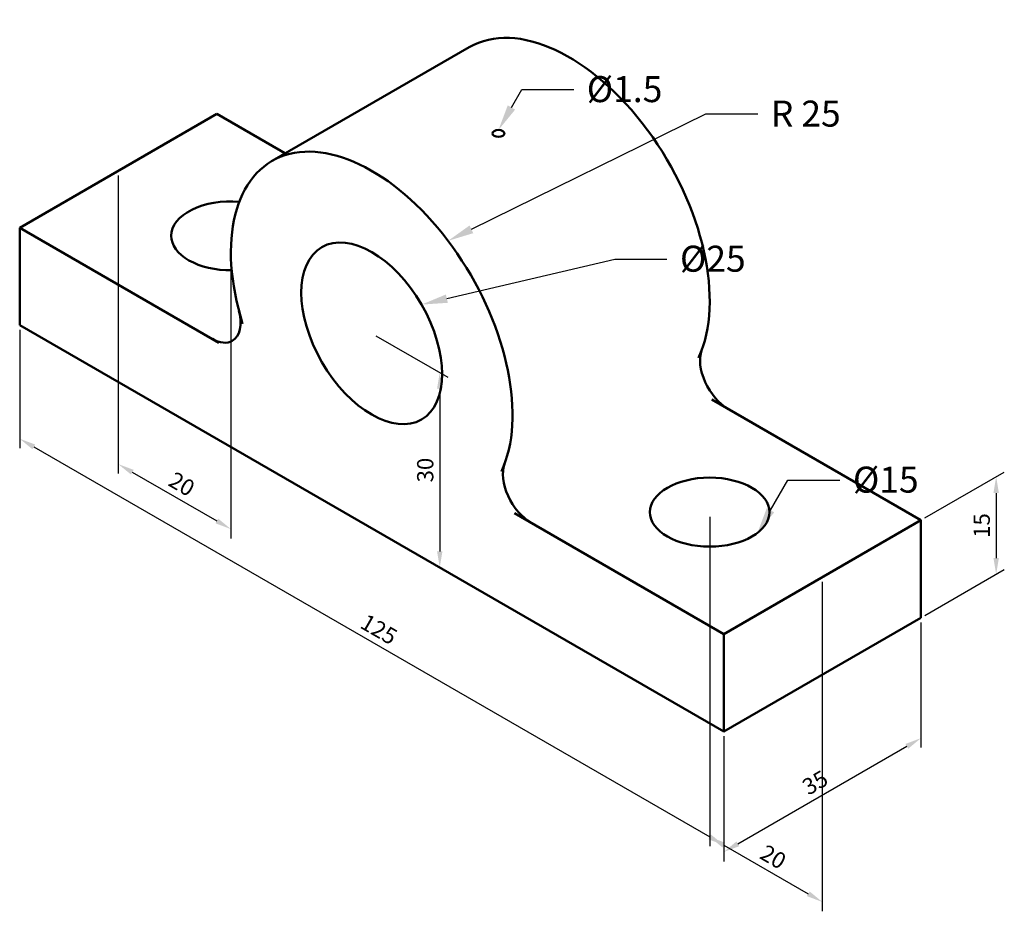
# Model space of a CAD drawing. Units: millimetres. Extents: x 2165 to 2316, y 1151 to 1289.
import ezdxf
from ezdxf import colors
from ezdxf.entities.mleader import LeaderData, LeaderLine
from ezdxf.math import Vec2, Vec3

# ---------------------------------------------------------------- set-up
doc = ezdxf.new("R2010")
doc.units = ezdxf.units.MM
for name, color, linetype, lineweight in [('M-DIMS', 2, 'Continuous', 25), ('M-OUTL', 7, 'Continuous', 50), ('M-TEXT', 3, 'Continuous', 25)]:
    doc.layers.add(name, color=color, linetype=linetype, lineweight=lineweight)
doc.styles.get("Standard").update_dxf_attribs({"font": 'arial.ttf'})
doc.dimstyles.new('ISO-25', dxfattribs={"dimtxt": 2.5, "dimasz": 2.5, "dimexe": 1.25, "dimexo": 0.625, "dimtad": 1, "dimtxsty": 'Standard', "dimcen": 2.5, "dimadec": 0, "dimazin": 0, "dimtfac": 1, "dimtmove": 0, "dimatfit": 3, "dimfxl": 1, "dimarcsym": 0})

# ---------------------------------------------------------------- blocks, each defined once
blk = doc.blocks.new('*D1')
at = {"layer": 'Defpoints', "color": 0, "transparency": 16777216}
for p in [(2164.55, 1241.65), (2272.81, 1179.15), (2272.81, 1161.69)]:
    blk.add_point(p, dxfattribs=at)
at = {"layer": 'M-DIMS', "color": 0, "lineweight": -2, "transparency": 16777216}
for p, q in [((2164.55, 1240.93), (2164.55, 1222.75)), ((2166.72, 1222.94), (2270.64, 1162.94)), ((2272.81, 1178.43), (2272.81, 1160.25))]:
    blk.add_line(p, q, dxfattribs=at)
at = {"layer": 'M-DIMS', "color": 0, "transparency": 16777216}
for points in [[(2166.93, 1223.3), (2166.51, 1222.58), (2164.55, 1224.19)], [(2270.85, 1163.3), (2270.43, 1162.58), (2272.81, 1161.69)]]:
    blk.add_solid(points, dxfattribs=at)
at = {"layer": 'M-DIMS', "color": 0, "transparency": 16777216, "insert": (2219.63, 1194.59), "char_height": 2.5, "attachment_point": 5, "rotation": 330}
blk.add_mtext('125', dxfattribs=at)
blk = doc.blocks.new('*D2')
at = {"layer": 'Defpoints', "color": 0, "transparency": 16777216}
for p in [(2303.12, 1196.65), (2272.81, 1179.15), (2303.12, 1178.13)]:
    blk.add_point(p, dxfattribs=at)
at = {"layer": 'M-DIMS', "color": 0, "lineweight": -2, "transparency": 16777216}
for p, q in [((2303.12, 1195.93), (2303.12, 1176.68)), ((2272.81, 1178.43), (2272.81, 1159.18)), ((2274.97, 1161.88), (2300.95, 1176.88))]:
    blk.add_line(p, q, dxfattribs=at)
at = {"layer": 'M-DIMS', "color": 0, "transparency": 16777216}
for points in [[(2300.74, 1177.24), (2301.16, 1176.51), (2303.12, 1178.13)], [(2274.76, 1162.24), (2275.18, 1161.51), (2272.81, 1160.63)]]:
    blk.add_solid(points, dxfattribs=at)
at = {"layer": 'M-DIMS', "color": 0, "transparency": 16777216, "insert": (2287.01, 1171.02), "char_height": 2.5, "attachment_point": 5, "rotation": 30}
blk.add_mtext('35', dxfattribs=at)
blk = doc.blocks.new('*D3')
at = {"layer": 'Defpoints', "color": 0, "transparency": 16777216}
for p in [(2303.12, 1211.65), (2314.69, 1203.34), (2303.12, 1196.65)]:
    blk.add_point(p, dxfattribs=at)
at = {"layer": 'M-DIMS', "color": 0, "lineweight": -2, "transparency": 16777216}
for p, q in [((2303.74, 1212.02), (2315.94, 1219.06)), ((2314.69, 1215.84), (2314.69, 1205.84)), ((2303.74, 1197.02), (2315.94, 1204.06))]:
    blk.add_line(p, q, dxfattribs=at)
at = {"layer": 'M-DIMS', "color": 0, "transparency": 16777216}
for points in [[(2314.27, 1215.84), (2315.11, 1215.84), (2314.69, 1218.34)], [(2314.27, 1205.84), (2315.11, 1205.84), (2314.69, 1203.34)]]:
    blk.add_solid(points, dxfattribs=at)
at = {"layer": 'M-DIMS', "color": 0, "transparency": 16777216, "insert": (2312.79, 1210.84), "char_height": 2.5, "attachment_point": 5, "rotation": 90}
blk.add_mtext('15', dxfattribs=at)
blk = doc.blocks.new('*D4')
at = {"layer": 'Defpoints', "color": 0, "transparency": 16777216}
for p in [(2179.71, 1265.4), (2197.03, 1255.4), (2197.03, 1210.29)]:
    blk.add_point(p, dxfattribs=at)
at = {"layer": 'M-DIMS', "color": 0, "lineweight": -2, "transparency": 16777216}
for p, q in [((2179.71, 1264.68), (2179.71, 1218.85)), ((2197.03, 1254.68), (2197.03, 1208.85)), ((2181.87, 1219.04), (2194.86, 1211.54))]:
    blk.add_line(p, q, dxfattribs=at)
at = {"layer": 'M-DIMS', "color": 0, "transparency": 16777216}
for points in [[(2182.08, 1219.4), (2181.67, 1218.68), (2179.71, 1220.29)], [(2195.07, 1211.9), (2194.66, 1211.18), (2197.03, 1210.29)]]:
    blk.add_solid(points, dxfattribs=at)
at = {"layer": 'M-DIMS', "color": 0, "transparency": 16777216, "insert": (2189.32, 1216.94), "char_height": 2.5, "attachment_point": 5, "rotation": 330}
blk.add_mtext('20', dxfattribs=at)
blk = doc.blocks.new('*D5')
at = {"layer": 'Defpoints', "color": 0, "transparency": 16777216}
for p in [(2270.64, 1212.9), (2287.96, 1202.9), (2287.96, 1152.94)]:
    blk.add_point(p, dxfattribs=at)
at = {"layer": 'M-DIMS', "color": 0, "lineweight": -2, "transparency": 16777216}
for p, q in [((2270.64, 1212.18), (2270.64, 1161.5)), ((2287.96, 1202.18), (2287.96, 1151.5)), ((2272.81, 1161.69), (2285.8, 1154.19))]:
    blk.add_line(p, q, dxfattribs=at)
at = {"layer": 'M-DIMS', "color": 0, "transparency": 16777216}
for points in [[(2273.01, 1162.05), (2272.6, 1161.33), (2270.64, 1162.94)], [(2286.01, 1154.55), (2285.59, 1153.83), (2287.96, 1152.94)]]:
    blk.add_solid(points, dxfattribs=at)
at = {"layer": 'M-DIMS', "color": 0, "transparency": 16777216, "insert": (2280.25, 1159.59), "char_height": 2.5, "attachment_point": 5, "rotation": 330}
blk.add_mtext('20', dxfattribs=at)
blk = doc.blocks.new('*D6')
at = {"layer": 'Defpoints', "color": 0, "transparency": 16777216}
for p in [(2218.68, 1240.4), (2218.68, 1210.4), (2229.14, 1204.37)]:
    blk.add_point(p, dxfattribs=at)
at = {"layer": 'M-DIMS', "color": 0, "lineweight": -2, "transparency": 16777216}
for p, q in [((2219.3, 1240.04), (2230.39, 1233.65)), ((2229.14, 1231.87), (2229.14, 1206.87)), ((2219.3, 1210.04), (2230.39, 1203.65))]:
    blk.add_line(p, q, dxfattribs=at)
at = {"layer": 'M-DIMS', "color": 0, "transparency": 16777216}
for points in [[(2228.72, 1231.87), (2229.55, 1231.87), (2229.14, 1234.37)], [(2228.72, 1206.87), (2229.55, 1206.87), (2229.14, 1204.37)]]:
    blk.add_solid(points, dxfattribs=at)
at = {"layer": 'M-DIMS', "color": 0, "transparency": 16777216, "insert": (2227.23, 1219.37), "char_height": 2.5, "attachment_point": 5, "rotation": 90}
blk.add_mtext('30', dxfattribs=at)

msp = doc.modelspace()

# ---------------------------------------------------------------- linework, layer by layer
at = {"layer": 'M-OUTL'}
for p, q in [((2203.37, 1266.921), (2233.681, 1284.421)), ((2194.864, 1274.154), (2164.553, 1256.654)), ((2205.689, 1267.904), (2194.864, 1274.154)), ((2164.553, 1256.654), (2164.553, 1241.654)), ((2164.553, 1256.654), (2195.197, 1238.962)), ((2164.553, 1241.654), (2272.806, 1179.154)), ((2303.117, 1211.654), (2270.966, 1230.217)), ((2272.806, 1194.154), (2240.655, 1212.717)), ((2303.117, 1211.654), (2272.806, 1194.154)), ((2303.117, 1196.654), (2303.117, 1211.654)), ((2272.806, 1179.154), (2303.117, 1196.654)), ((2272.806, 1194.154), (2272.806, 1179.154))]:
    msp.add_line(p, q, dxfattribs=at)
for centre, major_axis, start_param, end_param in [((2248.991, 1257.904), (15.309, -26.517), 6.6684627, 9.424778), ((2218.68, 1240.404), (15.309, -26.517), 6.6684627, 10.6214399), ((2197.029, 1255.404), (9.186, 0), 1.4300979, 3.1415927), ((2197.029, 1255.404), (9.186, 0), 3.1415927, 4.7264655), ((2194.185, 1244.546), (3.062, -5.303), 0, 1.1252351), ((2194.185, 1244.546), (3.062, -5.303), 5.4977871, 6.2831853), ((2273.486, 1233.762), (-3.062, 5.303), 0.4455613, 2.3561945), ((2243.175, 1216.262), (-3.062, 5.303), 0.4455613, 2.3561945)]:
    msp.add_ellipse(centre, major_axis=major_axis, ratio=0.5773503, start_param=start_param, end_param=end_param, dxfattribs=at)
for centre, major_axis in [((2238.164, 1271.151), (-0.919, 0)), ((2218.68, 1240.404), (7.655, -13.258)), ((2270.641, 1212.904), (-9.186, 0))]:
    msp.add_ellipse(centre, major_axis=major_axis, ratio=0.5773503, dxfattribs=at)

# ---------------------------------------------------------------- dimensions: what is measured, and where the dimension line sits
at = {"layer": 'M-DIMS'}
for p1, p2, distance, picture, middle in [((2179.709, 1265.404), (2197.029, 1255.404), -39.069, '*D4', (2189.32, 1216.938)), ((2164.553, 1241.654), (2272.806, 1179.154), -15.124, '*D1', (2219.63, 1194.587)), ((2270.641, 1212.904), (2287.962, 1202.904), -43.27, '*D5', (2280.252, 1159.587)), ((2272.806, 1179.154), (2303.117, 1196.654), -16.047, '*D2', (2287.011, 1171.023))]:
    dim = msp.add_aligned_dim(p1=p1, p2=p2, distance=distance, dimstyle='ISO-25', override={"dimclrd": 0, "dimclre": 0, "dimclrt": 0}, dxfattribs=at)
    dim.commit()
    dim.dimension.update_dxf_attribs({"geometry": picture, "text_midpoint": middle})
for base, p1, p2, picture, middle in [((2229.136, 1204.367), (2218.68, 1240.404), (2218.68, 1210.404), '*D6', (2227.234, 1219.367)), ((2314.69, 1203.336), (2303.117, 1211.654), (2303.117, 1196.654), '*D3', (2312.789, 1210.836))]:
    dim = msp.add_linear_dim(base=base, p1=p1, p2=p2, angle=90, dimstyle='ISO-25', override={"dimclrd": 0, "dimclre": 0, "dimclrt": 0}, dxfattribs=at)
    dim.commit()
    dim.dimension.update_dxf_attribs({"geometry": picture, "text_midpoint": middle})

# ---------------------------------------------------------------- leaders
at = {"layer": 'M-TEXT'}
ml = msp.add_multileader_mtext('Standard', dxfattribs=at)
ml.set_content('%%C1.5', color=256)
ml.set_leader_properties()
ml.build(insert=Vec2(0, 0))
ctx = ml.context
ctx.base_point, ctx.plane_origin = Vec3(2249.746, 1277.886), Vec3(2238.164, 1271.681)
notes = []
notes.append((ctx, [(0, (1, 1, 0), (2241.746, 1277.886), (1, 0), 8, [(0, [(2238.164, 1271.681)], 0, [])])]))
ctx.mtext.insert, ctx.mtext.flow_direction = Vec3(2251.746, 1279.967), 5
ml = msp.add_multileader_mtext('Standard', dxfattribs=at)
ml.set_content('R 25', color=256)
ml.set_leader_properties()
ml.build(insert=Vec2(0, 0))
ctx = ml.context
ctx.base_point, ctx.plane_origin = Vec3(2278.04, 1274.168), Vec3(2230.418, 1254.634)
notes.append((ctx, [(0, (1, 1, 0), (2270.04, 1274.168), (1, 0), 8, [(0, [(2230.418, 1254.634)], 0, [])])]))
ctx.mtext.insert, ctx.mtext.flow_direction = Vec3(2280.04, 1276.202), 5
ml = msp.add_multileader_mtext('Standard', dxfattribs=at)
ml.set_content('%%C25', color=256)
ml.set_leader_properties()
ml.build(insert=Vec2(0, 0))
ctx = ml.context
ctx.base_point, ctx.plane_origin = Vec3(2264.069, 1251.801), Vec3(2226.334, 1244.824)
notes.append((ctx, [(0, (1, 1, 0), (2256.069, 1251.801), (1, 0), 8, [(0, [(2226.334, 1244.824)], 0, [])])]))
ctx.mtext.insert, ctx.mtext.flow_direction = Vec3(2266.069, 1253.882), 5
ml = msp.add_multileader_mtext('Standard', dxfattribs=at)
ml.set_content('%%C15', color=256)
ml.set_leader_properties()
ml.build(insert=Vec2(0, 0))
ctx = ml.context
ctx.base_point, ctx.plane_origin = Vec3(2290.665, 1217.82), Vec3(2277.99, 1209.722)
notes.append((ctx, [(0, (1, 1, 0), (2282.665, 1217.82), (1, 0), 8, [(0, [(2277.99, 1209.722)], 0, [])])]))
ctx.mtext.insert, ctx.mtext.flow_direction = Vec3(2292.665, 1219.901), 5
for ctx, leaders in notes:
    for number, flags, end, landing, length, lines in leaders:
        leader = LeaderData()
        leader.index, (leader.has_last_leader_line, leader.has_dogleg_vector, leader.attachment_direction) = number, flags
        leader.last_leader_point, leader.dogleg_vector, leader.dogleg_length = Vec3(end), Vec3(landing), length
        for number, points, colour, breaks in lines:
            line = LeaderLine()
            line.index, line.vertices, line.color, line.breaks = number, Vec3.list(points), colors.encode_raw_color(colour), breaks
            leader.lines.append(line)
        ctx.leaders.append(leader)

doc.saveas('drawing.dxf')
